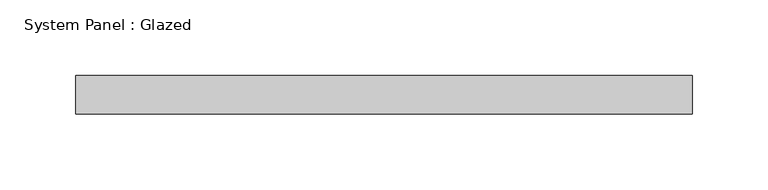
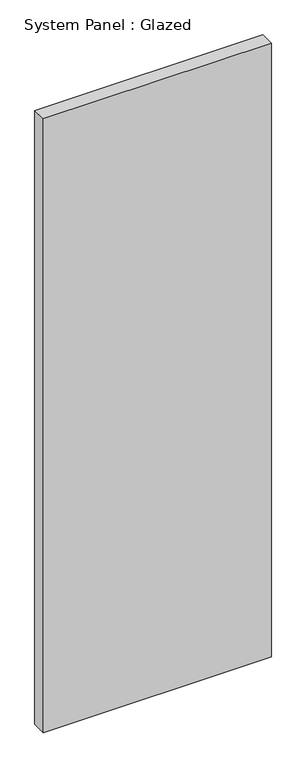
"""IFC4 building model written with IfcOpenShell, lengths in millimetres: plate geometry, System Panel : Glazed."""

from ifc_helpers import new_model, si_unit, origin, origin_with_axes, place, context, project, spatial, polyline, outline, extrude, source, transform, mapped, element, save


def system_panel_glazed_f1530dac(model_context):
    return source(origin(), model_context, "Body", "SweptSolid", [
        extrude(outline(polyline([(203.2, 19.05), (-203.2, 19.05), (-203.2, 44.45), (203.2, 44.45), (203.2, 19.05)])), origin_with_axes(), (0.0, 0.0, 1.0), 1155.7),
    ])


if __name__ == "__main__":
    model = new_model("IFC4")
    model_context = context("Model", 3, world=origin())
    ifc_project = project(units=[si_unit("LENGTHUNIT", "METRE", prefix="MILLI")], contexts=[model_context])
    site = spatial("IfcSite", under=ifc_project)
    building = spatial("IfcBuilding", under=site)
    placement = place(None, origin())
    system_panel_glazed_shape = system_panel_glazed_f1530dac(model_context)
    element("IfcPlate", 1, ObjectType="System Panel : Glazed", at=placement, inside=building, context=model_context, shape_type="MappedRepresentation", body=[
        mapped(system_panel_glazed_shape, transform((0.0, 0.0, 0.0), x_axis=(1.0, 0.0, 0.0), y_axis=(0.0, 1.0, 0.0), z_axis=(0.0, 0.0, 1.0))),
    ])
    save(model, "model.ifc")

# Revit data of these elements
# Type "System Panel : Glazed"
#   Construction Type Id = "GSP4R"
#   Analytic Construction = "1/8 in Pilkington single glazing"
#   Visual Light Transmittance = 0.9
#   Solar Heat Gain Coefficient = 0.86
#   Heat Transfer Coefficient (U) = 1.18115 BTU/(h·ft²·°F)
# Element 1 (IfcPlate, "System Panel : Glazed")
#   Materials on its faces: "Glass"
# Materials
#   "Glass": class "Glass", colour RGB 0 128 192, transparency 0.75, Description = "Soda Lime Glass", Cost = 0
